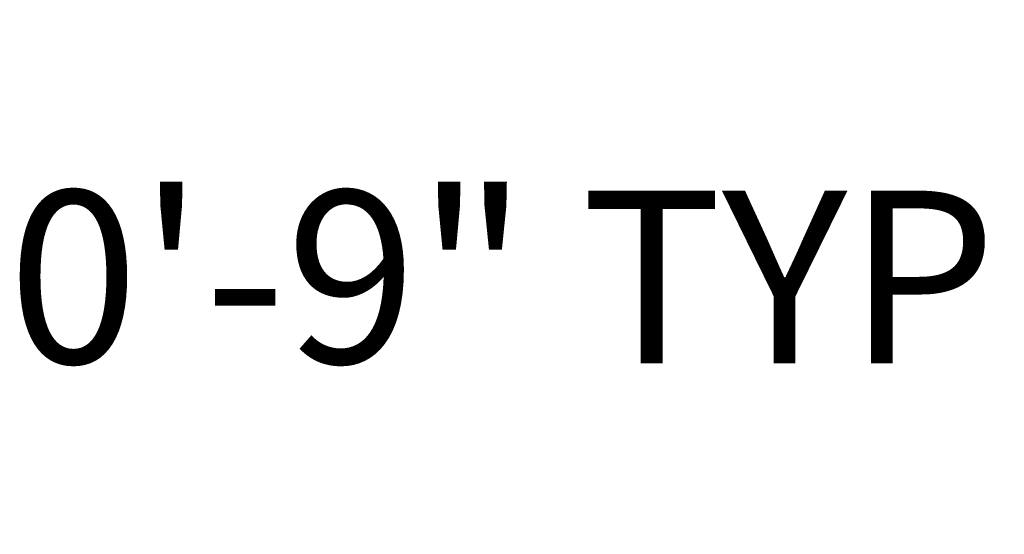
# Model space of a CAD drawing. Units: inches. Extents: x 29 to 6336, y 3 to 2592.
# Tile 2 of 8: x 5144 to 5288, y 2402 to 2477. Entities that reach past the tile are written whole.
import ezdxf

# ---------------------------------------------------------------- set-up
doc = ezdxf.new("R2010")
doc.units = ezdxf.units.IN
doc.header["$MEASUREMENT"] = 0
doc.layers.add('A-ANNO-DIMS', color=2, linetype='Continuous', lineweight=18)
doc.styles.get("Standard").update_dxf_attribs({"font": 'arial.ttf'})
doc.dimstyles.get("Standard").update_dxf_attribs({"dimtxt": 25.18, "dimasz": 25.18, "dimexe": 0.18, "dimexo": 0.0625, "dimgap": 0.09, "dimtad": 0, "dimtih": 1, "dimtoh": 1, "dimdec": 0, "dimzin": 0, "dimdsep": 46, "dimlunit": 3, "dimtxsty": 'Standard', "dimcen": 0.09, "dimadec": 0, "dimazin": 0, "dimtfac": 1, "dimtdec": 0, "dimtofl": 0, "dimtmove": 0, "dimatfit": 3, "dimfxl": 1, "dimtolj": 1, "dimtzin": 0, "dimarcsym": 0})

# ---------------------------------------------------------------- blocks, each defined once
blk = doc.blocks.new('*D23')
at = {"layer": 'A-ANNO-DIMS', "color": 0, "lineweight": -2, "transparency": 16777216}
for p, q in [((5321.48, 2439.75), (5296.3, 2439.75)), ((5346.66, 2432.01), (5346.66, 2439.93)), ((5355.66, 2432.01), (5355.66, 2439.93)), ((5380.84, 2439.75), (5406.02, 2439.75))]:
    blk.add_line(p, q, dxfattribs=at)
at = {"layer": 'A-ANNO-DIMS', "color": 0, "transparency": 16777216}
for points in [[(5321.48, 2443.94), (5321.48, 2435.55), (5346.66, 2439.75)], [(5380.84, 2443.94), (5380.84, 2435.55), (5355.66, 2439.75)]]:
    blk.add_solid(points, dxfattribs=at)
at = {"layer": 'Defpoints', "color": 0, "transparency": 16777216}
for p in [(5346.66, 2439.75), (5346.66, 2431.95), (5355.66, 2431.95)]:
    blk.add_point(p, dxfattribs=at)
at = {"layer": 'A-ANNO-DIMS', "color": 0, "transparency": 16777216, "insert": (5219.47, 2439.75), "char_height": 25.18, "attachment_point": 5}
blk.add_mtext('\\A1;0\'-9" TYP.', dxfattribs=at)

msp = doc.modelspace()

# ---------------------------------------------------------------- dimensions: what is measured, and where the dimension line sits
at = {"layer": 'A-ANNO-DIMS'}
dim = msp.add_linear_dim(base=(5346.66, 2439.75), p1=(5355.66, 2431.95), p2=(5346.66, 2431.95), angle=180, text='<> TYP.', dimstyle='Standard', override={"dimdec": 1, "dimlfac": 1, "dimrnd": 0, "dimzin": 1, "dimdsep": 46, "dimlunit": 4, "dimfrac": 2}, dxfattribs=at)
dim.commit()
dim.dimension.update_dxf_attribs({"geometry": '*D23', "text_midpoint": (5219.47, 2439.75)})

doc.saveas('drawing.dxf')
